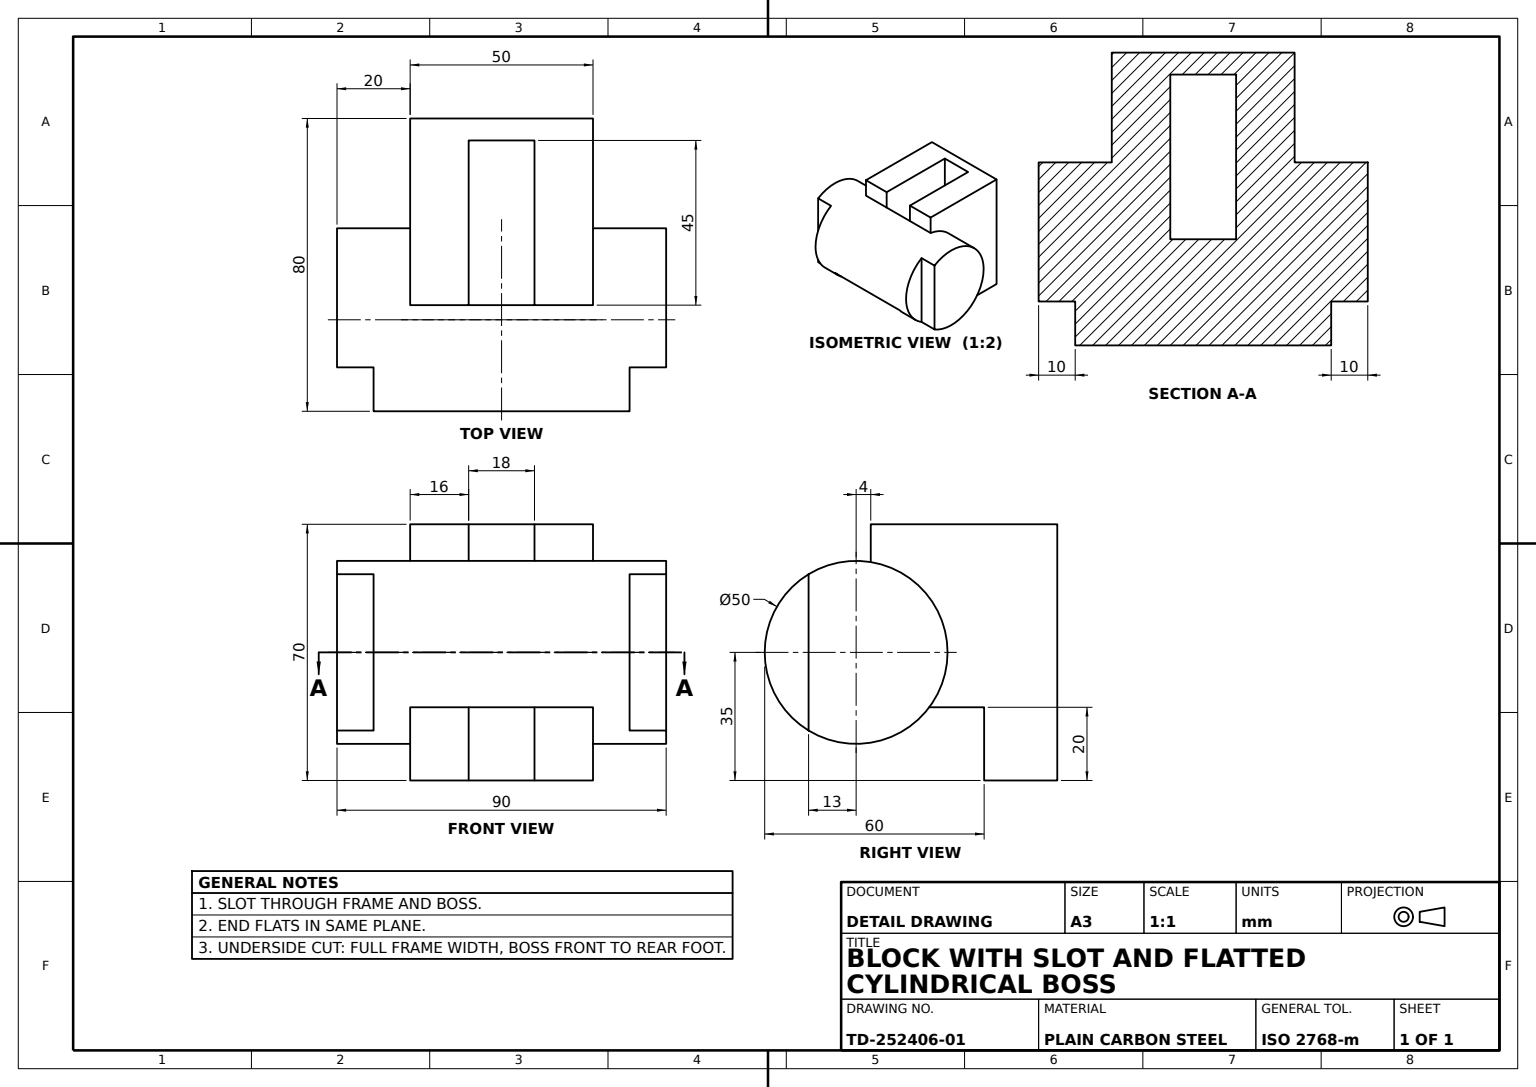
SolidWorks part; units mm, degrees
material "Plain Carbon Steel"
ref_plane "Front Plane" through (0, 0, 0) normal (0, 0, 1) x (1, 0, 0)
ref_plane "Top Plane" through (0, 0, 0) normal (0, 1, 0) x (1, 0, 0)
ref_plane "Right Plane" through (0, 0, 0) normal (1, 0, 0) x (0, 0, -1)
sketch "Base Plate Sketch" plane through (0, 0, 0) normal (0, 0, 1) x (1, 0, 0)
  line L0 (0, 0) -> (0, -70)
  line L1 (0, -70) -> (50, -70)
  line L2 (50, -70) -> (50, 0)
  line L3 (50, 0) -> (0, 0)
  dimension "D1" = 50
  dimension "D2" = 70
extrude "Base Plate" add sketch "Base Plate Sketch" along normal blind 9
sketch "U-Frame Sketch" plane through (0, -70, 0) normal (0, -1, 0) x (1, 0, 0)
  line L0 (0, 9) -> (0, 20)
  line L1 (0, 20) -> (16, 20)
  line L2 (16, 20) -> (16, 9)
  line L3 (0, 9) -> (50, 9) construction
  line L4 (0, 9) -> (16, 9)
  line L5 (50, 9) -> (50, 20)
  line L6 (50, 20) -> (34, 20)
  line L7 (34, 20) -> (34, 9)
  line L8 (34, 9) -> (50, 9)
  line L9 (50, 9) -> (50, 0) construction
  line L10 (0, 0) -> (50, 0) construction
  dimension "D1" = 16
  dimension "D2" = 20
extrude "U-Frame" add sketch "U-Frame Sketch" against normal blind 70
sketch "Side Block A Sketch" plane through (0, 0, 0) normal (-1, 0, 0) x (0, 0, 1)
  line L0 (20, 0) -> (54, 0)
  line L1 (54, 0) -> (54, -50)
  line L2 (54, -50) -> (20, -50)
  line L3 (20, 0) -> (20, -70) construction
  line L4 (20, -50) -> (20, 0)
  line L5 (0, 0) -> (0, -70) construction
  line L6 (20, -70) -> (0, -70) construction
  dimension "D1" = 54
  dimension "D2" = 20
extrude "Side Block A" add sketch "Side Block A Sketch" against normal blind 16
sketch "Side Block B Sketch" plane through (50, 0, 0) normal (1, 0, 0) x (0, 0, -1)
  line L0 (-20, 0) -> (-54, 0)
  line L1 (-54, 0) -> (-54, -50)
  line L2 (-54, -50) -> (-20, -50)
  line L3 (-20, -50) -> (-20, 0)
extrude "Side Block B" add sketch "Side Block B Sketch" against normal blind 16
sketch "Base Recess Sketch" plane through (0, 0, 0) normal (0, 0, -1) x (-1, 0, 0)
  line L1 (-50, 0) -> (0, 0)
  line L2 (-50, 0) -> (-50, -70)
  line L3 (-50, -70) -> (0, -70)
  line L4 (0, 0) -> (0, -70)
extrude "Base Recess Cut" cut sketch "Base Recess Sketch" against normal blind 3
sketch "Top Lip Sketch" plane through (0, 0, 20) normal (0, 0, 1) x (1, 0, 0)
  line L0 (0, -50) -> (16, -50)
  line L1 (16, -50) -> (16, -70)
  line L2 (16, -70) -> (0, -70)
  line L3 (0, -70) -> (0, -50)
  line L4 (34, -50) -> (50, -50)
  line L5 (50, -50) -> (50, -70)
  line L6 (50, -70) -> (34, -70)
  line L7 (34, -70) -> (34, -50)
extrude "Top Lip" add sketch "Top Lip Sketch" along normal blind 3
sketch "Cylinder Sketch" plane through (0, 0, 0) normal (-1, 0, 0) x (0, 0, 1)
  line L0 (23, -70) -> (3, -70) construction
  circle A0 centre (58, -35) radius 25
  dimension "D1" = 50
  dimension "D2" = 50
  dimension "D3" = 4
  dimension "D4" = 35
extrude "Cylinder Ø50" add sketch "Cylinder Sketch" against normal blind 70
sketch "Cylinder Extension Sketch" plane through (0, 0, 0) normal (-1, 0, 0) x (0, 0, 1)
  circle A0 centre (58, -35) radius 25
  dimension "D1" = 50
  dimension "D2" = 50
extrude "Cylinder Extension Ø50" add sketch "Cylinder Extension Sketch" along normal blind 20
sketch "U-Slot Sketch" plane through (0, 0, 23) normal (0, 0, 1) x (1, 0, 0)
  line L0 (34, -70) -> (50, -70)
  line L1 (50, -70) -> (50, -50)
  line L2 (50, -50) -> (0, -50)
  line L3 (0, -50) -> (0, -70)
  line L4 (0, -70) -> (34, -70)
  line L6 (34, -70) -> (50, -70) construction
  dimension "D1" = 20
extrude "U-Slot Cut" cut sketch "U-Slot Sketch" along normal blind 60
sketch "Frame Clearance Sketch" plane through (0, -50, 0) normal (0, -1, 0) x (1, 0, 0)
  line L0 (16, 33) -> (16, 54)
  line L1 (16, 33) -> (16, 54) construction
  line L2 (16, 54) -> (34, 54)
  line L3 (34, 54) -> (34, 33)
  line L4 (34, 33) -> (16, 33)
  line L5 (16, 33) -> (34, 33) construction
  line L7 (34, 38) -> (16, 38) construction
  dimension "D1" = 16
extrude "Frame Clearance Cut" cut sketch "Frame Clearance Sketch" against normal blind 50
sketch "End Flat A Sketch" plane through (-20, 0, 0) normal (-1, 0, 0) x (0, 0, 1)
  line L1 (71, -35) -> (71, -13.6458)
  line L2 (71, -13.6458) -> (71, -56.3542)
  circle A1 centre (58, -35) radius 25 construction
  arc A2 (71, -56.3542) -> (71, -13.6458) centre (58, -35) ccw
  circle M1 centre (58, -35) radius 25
  dimension "D1" = 50
  dimension "D2" = 13
extrude "End Flat A" cut sketch "End Flat A Sketch" against normal blind 10 contours L1 L2 M1
sketch "End Flat B Sketch" plane through (70, 0, 0) normal (1, 0, 0) x (0, 0, -1)
  line L1 (-71, -35) -> (-71, -13.6458)
  line L2 (-71, -13.6458) -> (-71, -56.3542)
  circle A0 centre (-58, -35) radius 25 construction
  arc A2 (-71, -13.6458) -> (-71, -56.3542) centre (-58, -35) ccw
  circle M1 centre (-58, -35) radius 25
  dimension "D1" = 50
  dimension "D2" = 25
  dimension "D3" = 13
extrude "End Flat B" cut sketch "End Flat B Sketch" against normal blind 10 contours L2 L1 M1
